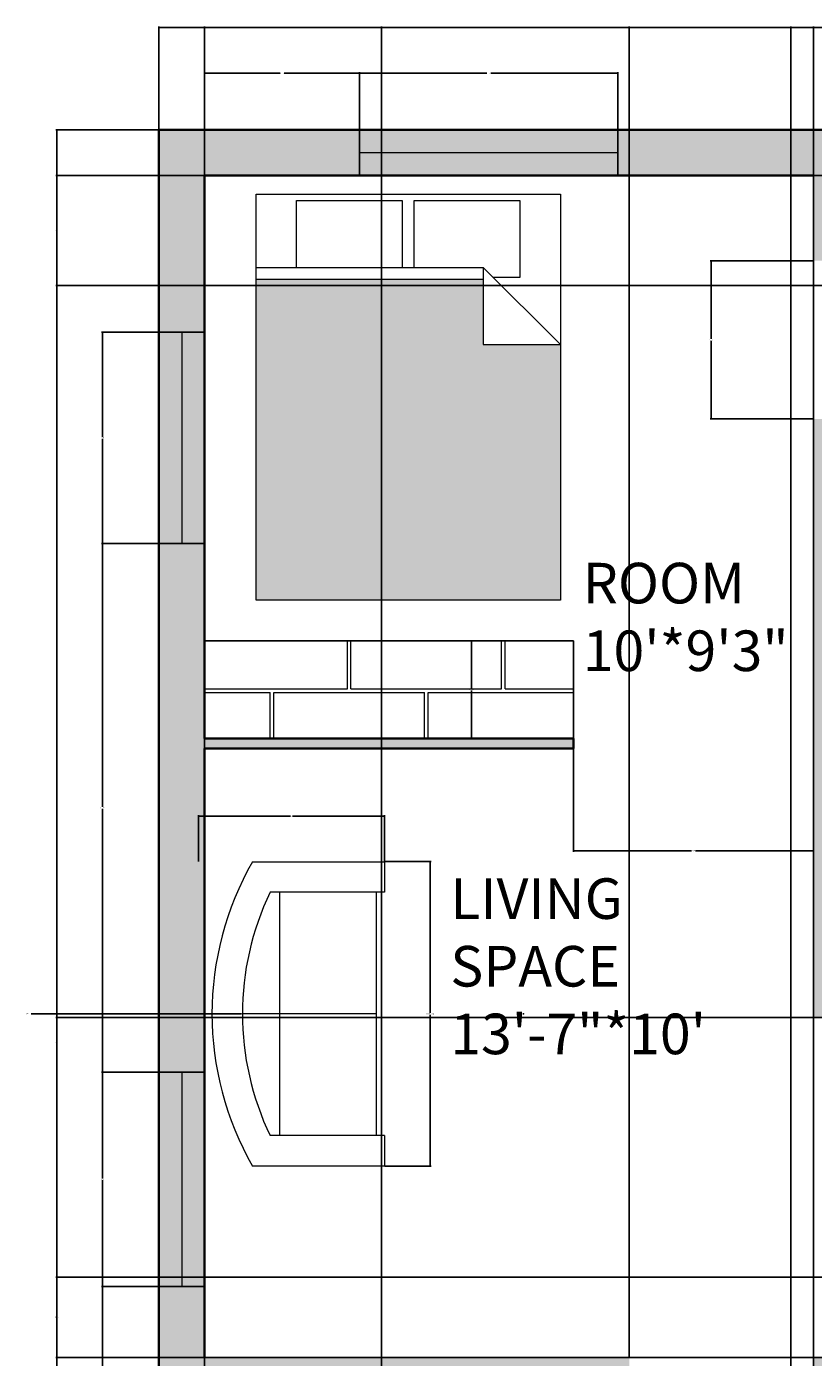
# Model space of a CAD drawing. Units: inches. Extents: x 17031430 to 17032061, y 16082759 to 16083238.
# Tile 2 of 3: x 17031430 to 17031585, y 16082898 to 16083160. Entities that reach past the tile are written whole.
import ezdxf

# ---------------------------------------------------------------- set-up
doc = ezdxf.new("R2010")
doc.units = ezdxf.units.IN
doc.header["$MEASUREMENT"] = 0
for name, color, linetype, lineweight in [('A-ANNO-DIMS', 2, 'Continuous', 18), ('A-AREA-IDEN', 7, 'Continuous', 25), ('A-FLOR-CASE', 8, 'Continuous', 25), ('A-FURN', 8, 'Continuous', 18), ('A-GLAZ', 4, 'Continuous', 18), ('A-WALL', 7, 'Continuous', 35)]:
    doc.layers.add(name, color=color, linetype=linetype, lineweight=lineweight)
for name, color, linetype, lineweight, true_color in [('A-FLOR-CASE-PATT', 9, 'Continuous', 13, 0xc7c8ca), ('A-GLAZ-PATT', 252, 'Continuous', 13, 0x939598), ('A-WALL-PATT', 18, 'Continuous', 13, 0x000000)]:
    doc.layers.add(name, color=color, linetype=linetype, lineweight=lineweight, true_color=true_color)
doc.styles.get("Standard").update_dxf_attribs({"font": 'arial.ttf'})
doc.dimstyles.get("Standard").update_dxf_attribs({"dimtxt": 0.18, "dimasz": 0.18, "dimexe": 0.18, "dimexo": 0.0625, "dimgap": 0.09, "dimtad": 0, "dimtih": 1, "dimtoh": 1, "dimdec": 0, "dimzin": 0, "dimdsep": 46, "dimlunit": 3, "dimtxsty": 'Standard', "dimcen": 0.09, "dimadec": 0, "dimazin": 0, "dimtfac": 1, "dimtdec": 0, "dimtofl": 0, "dimtmove": 0, "dimatfit": 3, "dimfxl": 1, "dimtolj": 1, "dimtzin": 0, "dimarcsym": 0})

# ---------------------------------------------------------------- blocks, each defined once
blk = doc.blocks.new('Bed - Queen')
for p, q in [((0, -80.00003), (0, 0)), ((0, 0), (59.99999, 0)), ((59.99999, 0), (59.99999, -80.00003)), ((7.99999, -1.2), (28.79998, -1.2)), ((7.99999, -14.4), (7.99999, -1.2)), ((28.79998, -1.2), (28.79998, -14.4)), ((31.19999, -1.2), (51.99999, -1.2)), ((31.19999, -14.4), (31.19999, -1.2)), ((51.99999, -1.2), (51.99999, -16.4)), ((0, -14.4), (44.8, -14.4)), ((59.99999, -29.6), (44.8, -14.4)), ((44.8, -14.4), (44.8, -29.6)), ((44.8, -16.8), (0, -16.8)), ((51.99999, -16.4), (46.79936, -16.4)), ((44.8, -29.6), (59.99999, -29.6)), ((59.99999, -80.00003), (0, -80.00003))]:
    blk.add_line(p, q)
blk = doc.blocks.new('Sofa - Roundback Loveseat 5 ft.')
for p, q in [((0, -32.44198), (0, -5.99998)), ((-24, -33.99998), (-24, -11.46958)), ((24.00004, -33.99998), (24.00004, -11.46958)), ((-23.9998, -13.38178), (23.99986, -13.38178)), ((-24, -32.44198), (24.00004, -32.44198))]:
    blk.add_line(p, q)
for points in [[(-24, -33.99998), (-30, -33.99998), (-30, -7.99998)], [(30.00004, -7.99998), (30.00004, -33.99998), (24.00004, -33.99998)]]:
    blk.add_lwpolyline(points)
for centre, radius, start, end in [((0, -60.24998), 60.24998, 60.13715, 119.8628), ((0, -61.38438), 55.38444, 64.32083, 115.6792)]:
    blk.add_arc(centre, radius, start, end)
blk = doc.blocks.new('*D10')
at = {"layer": 'A-ANNO-DIMS', "color": 0, "lineweight": -2, "transparency": 16777216}
for p, q in [((17031500.27, 16082995.46), (17031509.39, 16082995.46)), ((17031509.21, 16082995.28), (17031509.21, 16082965.64)), ((17031509.21, 16082935.64), (17031509.21, 16082965.28)), ((17031500.27, 16082935.46), (17031509.39, 16082935.46))]:
    blk.add_line(p, q, dxfattribs=at)
at = {"layer": 'A-ANNO-DIMS', "color": 0, "transparency": 16777216}
for points in [[(17031509.18, 16082995.28), (17031509.24, 16082995.28), (17031509.21, 16082995.46)], [(17031509.18, 16082935.64), (17031509.24, 16082935.64), (17031509.21, 16082935.46)]]:
    blk.add_solid(points, dxfattribs=at)
at = {"layer": 'Defpoints', "color": 0, "transparency": 16777216}
for p in [(17031500.21, 16082995.46), (17031509.21, 16082995.46), (17031500.21, 16082935.46)]:
    blk.add_point(p, dxfattribs=at)
at = {"layer": 'A-ANNO-DIMS', "color": 0, "transparency": 16777216, "insert": (17031509.21, 16082965.46), "char_height": 0.18, "attachment_point": 5}
blk.add_mtext('\\A1;LOVESEAT 60', dxfattribs=at)
blk = doc.blocks.new('*D11')
at = {"layer": 'A-ANNO-DIMS', "color": 0, "lineweight": -2, "transparency": 16777216}
for p, q in [((17031463.54, 16082995.52), (17031463.54, 16083004.64)), ((17031463.72, 16083004.46), (17031481.66, 16083004.46)), ((17031500.03, 16083004.46), (17031482.09, 16083004.46)), ((17031500.21, 16082995.52), (17031500.21, 16083004.64))]:
    blk.add_line(p, q, dxfattribs=at)
at = {"layer": 'A-ANNO-DIMS', "color": 0, "transparency": 16777216}
for points in [[(17031463.72, 16083004.49), (17031463.72, 16083004.43), (17031463.54, 16083004.46)], [(17031500.03, 16083004.49), (17031500.03, 16083004.43), (17031500.21, 16083004.46)]]:
    blk.add_solid(points, dxfattribs=at)
at = {"layer": 'Defpoints', "color": 0, "transparency": 16777216}
for p in [(17031463.54, 16083004.46), (17031463.54, 16082995.46), (17031500.21, 16082995.46)]:
    blk.add_point(p, dxfattribs=at)
at = {"layer": 'A-ANNO-DIMS', "color": 0, "transparency": 16777216, "insert": (17031481.88, 16083004.46), "char_height": 0.18, "attachment_point": 5}
blk.add_mtext('\\A1;37', dxfattribs=at)
blk = doc.blocks.new('*D14')
at = {"layer": 'A-ANNO-DIMS', "color": 0, "lineweight": -2, "transparency": 16777216}
for p, q in [((17031455.76, 16083139.8), (17031455.76, 16083160.07)), ((17031455.94, 16083159.89), (17031575.47, 16083159.89)), ((17031695.58, 16083159.89), (17031576.05, 16083159.89)), ((17031695.76, 16083139.8), (17031695.76, 16083160.07))]:
    blk.add_line(p, q, dxfattribs=at)
at = {"layer": 'A-ANNO-DIMS', "color": 0, "transparency": 16777216}
for points in [[(17031455.94, 16083159.92), (17031455.94, 16083159.86), (17031455.76, 16083159.89)], [(17031695.58, 16083159.92), (17031695.58, 16083159.86), (17031695.76, 16083159.89)]]:
    blk.add_solid(points, dxfattribs=at)
at = {"layer": 'Defpoints', "color": 0, "transparency": 16777216}
for p in [(17031695.76, 16083159.89), (17031455.76, 16083139.74), (17031695.76, 16083139.74)]:
    blk.add_point(p, dxfattribs=at)
at = {"layer": 'A-ANNO-DIMS', "color": 0, "transparency": 16777216, "insert": (17031575.76, 16083159.89), "char_height": 0.18, "attachment_point": 5}
blk.add_mtext('\\A1;240', dxfattribs=at)
blk = doc.blocks.new('*D15')
at = {"layer": 'A-ANNO-DIMS', "color": 0, "lineweight": -2, "transparency": 16777216}
for p, q in [((17031455.69, 16083139.74), (17031435.43, 16083139.74)), ((17031435.61, 16083139.56), (17031435.61, 16082959.92)), ((17031435.61, 16082779.92), (17031435.61, 16082959.56)), ((17031455.69, 16082779.74), (17031435.43, 16082779.74))]:
    blk.add_line(p, q, dxfattribs=at)
at = {"layer": 'A-ANNO-DIMS', "color": 0, "transparency": 16777216}
for points in [[(17031435.58, 16083139.56), (17031435.64, 16083139.56), (17031435.61, 16083139.74)], [(17031435.58, 16082779.92), (17031435.64, 16082779.92), (17031435.61, 16082779.74)]]:
    blk.add_solid(points, dxfattribs=at)
at = {"layer": 'Defpoints', "color": 0, "transparency": 16777216}
for p in [(17031435.61, 16083139.74), (17031455.76, 16083139.74), (17031455.76, 16082779.74)]:
    blk.add_point(p, dxfattribs=at)
at = {"layer": 'A-ANNO-DIMS', "color": 0, "transparency": 16777216, "insert": (17031435.61, 16082959.74), "char_height": 0.18, "attachment_point": 5}
blk.add_mtext('\\A1;360', dxfattribs=at)
blk = doc.blocks.new('*D16')
at = {"layer": 'A-ANNO-DIMS', "color": 0, "lineweight": -2, "transparency": 16777216}
for p, q in [((17031464.76, 16083130.8), (17031464.76, 16083151.07)), ((17031464.94, 16083150.89), (17031479.63, 16083150.89)), ((17031495.11, 16083150.89), (17031480.42, 16083150.89)), ((17031495.29, 16083130.8), (17031495.29, 16083151.07))]:
    blk.add_line(p, q, dxfattribs=at)
at = {"layer": 'A-ANNO-DIMS', "color": 0, "transparency": 16777216}
for points in [[(17031464.94, 16083150.92), (17031464.94, 16083150.86), (17031464.76, 16083150.89)], [(17031495.11, 16083150.92), (17031495.11, 16083150.86), (17031495.29, 16083150.89)]]:
    blk.add_solid(points, dxfattribs=at)
at = {"layer": 'Defpoints', "color": 0, "transparency": 16777216}
for p in [(17031495.29, 16083150.89), (17031464.76, 16083130.74), (17031495.29, 16083130.74)]:
    blk.add_point(p, dxfattribs=at)
at = {"layer": 'A-ANNO-DIMS', "color": 0, "transparency": 16777216, "insert": (17031480.02, 16083150.89), "char_height": 0.18, "attachment_point": 5}
blk.add_mtext('\\A1;30.53', dxfattribs=at)
blk = doc.blocks.new('*D17')
at = {"layer": 'A-ANNO-DIMS', "color": 0, "lineweight": -2, "transparency": 16777216}
for p, q in [((17031495.29, 16083130.8), (17031495.29, 16083151.07)), ((17031495.47, 16083150.89), (17031520.36, 16083150.89)), ((17031546.04, 16083150.89), (17031521.15, 16083150.89)), ((17031546.22, 16083130.8), (17031546.22, 16083151.07))]:
    blk.add_line(p, q, dxfattribs=at)
at = {"layer": 'A-ANNO-DIMS', "color": 0, "transparency": 16777216}
for points in [[(17031495.47, 16083150.92), (17031495.47, 16083150.86), (17031495.29, 16083150.89)], [(17031546.04, 16083150.92), (17031546.04, 16083150.86), (17031546.22, 16083150.89)]]:
    blk.add_solid(points, dxfattribs=at)
at = {"layer": 'Defpoints', "color": 0, "transparency": 16777216}
for p in [(17031546.22, 16083150.89), (17031495.29, 16083130.74), (17031546.22, 16083130.74)]:
    blk.add_point(p, dxfattribs=at)
at = {"layer": 'A-ANNO-DIMS', "color": 0, "transparency": 16777216, "insert": (17031520.76, 16083150.89), "char_height": 0.18, "attachment_point": 5}
blk.add_mtext('\\A1;50.94', dxfattribs=at)
blk = doc.blocks.new('*D23')
at = {"layer": 'A-ANNO-DIMS', "color": 0, "lineweight": -2, "transparency": 16777216}
for p, q in [((17031464.69, 16082911.7), (17031444.43, 16082911.7)), ((17031444.61, 16082911.52), (17031444.61, 16082887.51)), ((17031444.61, 16082863.13), (17031444.61, 16082887.14)), ((17031464.69, 16082862.95), (17031444.43, 16082862.95))]:
    blk.add_line(p, q, dxfattribs=at)
at = {"layer": 'A-ANNO-DIMS', "color": 0, "transparency": 16777216}
for points in [[(17031444.58, 16082911.52), (17031444.64, 16082911.52), (17031444.61, 16082911.7)], [(17031444.58, 16082863.13), (17031444.64, 16082863.13), (17031444.61, 16082862.95)]]:
    blk.add_solid(points, dxfattribs=at)
at = {"layer": 'Defpoints', "color": 0, "transparency": 16777216}
for p in [(17031444.61, 16082911.7), (17031464.76, 16082911.7), (17031464.76, 16082862.95)]:
    blk.add_point(p, dxfattribs=at)
at = {"layer": 'A-ANNO-DIMS', "color": 0, "transparency": 16777216, "insert": (17031444.61, 16082887.33), "char_height": 0.18, "attachment_point": 5}
blk.add_mtext('\\A1;48.74', dxfattribs=at)
blk = doc.blocks.new('*D24')
at = {"layer": 'A-ANNO-DIMS', "color": 0, "lineweight": -2, "transparency": 16777216}
for p, q in [((17031464.69, 16082953.98), (17031444.43, 16082953.98)), ((17031444.61, 16082953.8), (17031444.61, 16082933.02)), ((17031444.61, 16082911.88), (17031444.61, 16082932.66)), ((17031464.69, 16082911.7), (17031444.43, 16082911.7))]:
    blk.add_line(p, q, dxfattribs=at)
at = {"layer": 'A-ANNO-DIMS', "color": 0, "transparency": 16777216}
for points in [[(17031444.58, 16082953.8), (17031444.64, 16082953.8), (17031444.61, 16082953.98)], [(17031444.58, 16082911.88), (17031444.64, 16082911.88), (17031444.61, 16082911.7)]]:
    blk.add_solid(points, dxfattribs=at)
at = {"layer": 'Defpoints', "color": 0, "transparency": 16777216}
for p in [(17031444.61, 16082953.98), (17031464.76, 16082953.98), (17031464.76, 16082911.7)]:
    blk.add_point(p, dxfattribs=at)
at = {"layer": 'A-ANNO-DIMS', "color": 0, "transparency": 16777216, "insert": (17031444.61, 16082932.84), "char_height": 0.18, "attachment_point": 5}
blk.add_mtext('\\A1;42.28', dxfattribs=at)
blk = doc.blocks.new('*D25')
at = {"layer": 'A-ANNO-DIMS', "color": 0, "lineweight": -2, "transparency": 16777216}
for p, q in [((17031464.69, 16083058.17), (17031444.43, 16083058.17)), ((17031444.61, 16083057.99), (17031444.61, 16083006.26)), ((17031444.61, 16082954.16), (17031444.61, 16083005.89)), ((17031464.69, 16082953.98), (17031444.43, 16082953.98))]:
    blk.add_line(p, q, dxfattribs=at)
at = {"layer": 'A-ANNO-DIMS', "color": 0, "transparency": 16777216}
for points in [[(17031444.58, 16083057.99), (17031444.64, 16083057.99), (17031444.61, 16083058.17)], [(17031444.58, 16082954.16), (17031444.64, 16082954.16), (17031444.61, 16082953.98)]]:
    blk.add_solid(points, dxfattribs=at)
at = {"layer": 'Defpoints', "color": 0, "transparency": 16777216}
for p in [(17031444.61, 16083058.17), (17031464.76, 16083058.17), (17031464.76, 16082953.98)]:
    blk.add_point(p, dxfattribs=at)
at = {"layer": 'A-ANNO-DIMS', "color": 0, "transparency": 16777216, "insert": (17031444.61, 16083006.07), "char_height": 0.18, "attachment_point": 5}
blk.add_mtext('\\A1;104.19', dxfattribs=at)
blk = doc.blocks.new('*D26')
at = {"layer": 'A-ANNO-DIMS', "color": 0, "lineweight": -2, "transparency": 16777216}
for p, q in [((17031464.69, 16083099.83), (17031444.43, 16083099.83)), ((17031444.61, 16083099.65), (17031444.61, 16083079.18)), ((17031444.61, 16083058.35), (17031444.61, 16083078.82)), ((17031464.69, 16083058.17), (17031444.43, 16083058.17))]:
    blk.add_line(p, q, dxfattribs=at)
at = {"layer": 'A-ANNO-DIMS', "color": 0, "transparency": 16777216}
for points in [[(17031444.58, 16083099.65), (17031444.64, 16083099.65), (17031444.61, 16083099.83)], [(17031444.58, 16083058.35), (17031444.64, 16083058.35), (17031444.61, 16083058.17)]]:
    blk.add_solid(points, dxfattribs=at)
at = {"layer": 'Defpoints', "color": 0, "transparency": 16777216}
for p in [(17031444.61, 16083099.83), (17031464.76, 16083099.83), (17031464.76, 16083058.17)]:
    blk.add_point(p, dxfattribs=at)
at = {"layer": 'A-ANNO-DIMS', "color": 0, "transparency": 16777216, "insert": (17031444.61, 16083079), "char_height": 0.18, "attachment_point": 5}
blk.add_mtext('\\A1;41.66', dxfattribs=at)
blk = doc.blocks.new('*D38')
at = {"layer": 'A-ANNO-DIMS', "color": 0, "lineweight": -2, "transparency": 16777216}
for p, q in [((17031537.5, 16083017.68), (17031537.5, 16082997.41)), ((17031584.76, 16083017.68), (17031584.76, 16082997.41)), ((17031537.68, 16082997.59), (17031560.73, 16082997.59)), ((17031584.58, 16082997.59), (17031561.53, 16082997.59))]:
    blk.add_line(p, q, dxfattribs=at)
at = {"layer": 'A-ANNO-DIMS', "color": 0, "transparency": 16777216}
for points in [[(17031537.68, 16082997.62), (17031537.68, 16082997.56), (17031537.5, 16082997.59)], [(17031584.58, 16082997.62), (17031584.58, 16082997.56), (17031584.76, 16082997.59)]]:
    blk.add_solid(points, dxfattribs=at)
at = {"layer": 'Defpoints', "color": 0, "transparency": 16777216}
for p in [(17031537.5, 16083017.74), (17031584.76, 16083017.74), (17031537.5, 16082997.59)]:
    blk.add_point(p, dxfattribs=at)
at = {"layer": 'A-ANNO-DIMS', "color": 0, "transparency": 16777216, "insert": (17031561.13, 16082997.59), "char_height": 0.18, "attachment_point": 5}
blk.add_mtext('\\A1;47.26', dxfattribs=at)
blk = doc.blocks.new('*D39')
at = {"layer": 'A-ANNO-DIMS', "color": 0, "lineweight": -2, "transparency": 16777216}
for p, q in [((17031548.47, 16082897.8), (17031548.47, 16083160.07)), ((17031548.65, 16083159.89), (17031566.22, 16083159.89)), ((17031584.58, 16083159.89), (17031567.01, 16083159.89)), ((17031584.76, 16082897.8), (17031584.76, 16083160.07))]:
    blk.add_line(p, q, dxfattribs=at)
at = {"layer": 'A-ANNO-DIMS', "color": 0, "transparency": 16777216}
for points in [[(17031548.65, 16083159.92), (17031548.65, 16083159.86), (17031548.47, 16083159.89)], [(17031584.58, 16083159.92), (17031584.58, 16083159.86), (17031584.76, 16083159.89)]]:
    blk.add_solid(points, dxfattribs=at)
at = {"layer": 'Defpoints', "color": 0, "transparency": 16777216}
for p in [(17031584.76, 16083159.89), (17031548.47, 16082897.74), (17031584.76, 16082897.74)]:
    blk.add_point(p, dxfattribs=at)
at = {"layer": 'A-ANNO-DIMS', "color": 0, "transparency": 16777216, "insert": (17031566.61, 16083159.89), "char_height": 0.18, "attachment_point": 5}
blk.add_mtext('\\A1;36.29', dxfattribs=at)
blk = doc.blocks.new('*D41')
at = {"layer": 'A-ANNO-DIMS', "color": 0, "lineweight": -2, "transparency": 16777216}
for p, q in [((17031584.69, 16083113.92), (17031564.43, 16083113.92)), ((17031564.61, 16083113.74), (17031564.61, 16083098.51)), ((17031564.61, 16083082.92), (17031564.61, 16083098.15)), ((17031584.69, 16083082.74), (17031564.43, 16083082.74))]:
    blk.add_line(p, q, dxfattribs=at)
at = {"layer": 'A-ANNO-DIMS', "color": 0, "transparency": 16777216}
for points in [[(17031564.58, 16083113.74), (17031564.64, 16083113.74), (17031564.61, 16083113.92)], [(17031564.58, 16083082.92), (17031564.64, 16083082.92), (17031564.61, 16083082.74)]]:
    blk.add_solid(points, dxfattribs=at)
at = {"layer": 'Defpoints', "color": 0, "transparency": 16777216}
for p in [(17031564.61, 16083113.92), (17031584.76, 16083113.92), (17031584.76, 16083082.74)]:
    blk.add_point(p, dxfattribs=at)
at = {"layer": 'A-ANNO-DIMS', "color": 0, "transparency": 16777216, "insert": (17031564.61, 16083098.33), "char_height": 0.18, "attachment_point": 5}
blk.add_mtext('\\A1;31.176', dxfattribs=at)
blk = doc.blocks.new('*D44')
at = {"layer": 'A-ANNO-DIMS', "color": 0, "lineweight": -2, "transparency": 16777216}
for p, q in [((17031630.06, 16082964.74), (17031435.43, 16082964.74)), ((17031435.61, 16082964.56), (17031435.61, 16082931.42)), ((17031435.61, 16082897.92), (17031435.61, 16082931.06)), ((17031629.85, 16082897.74), (17031435.43, 16082897.74))]:
    blk.add_line(p, q, dxfattribs=at)
at = {"layer": 'A-ANNO-DIMS', "color": 0, "transparency": 16777216}
for points in [[(17031435.58, 16082964.56), (17031435.64, 16082964.56), (17031435.61, 16082964.74)], [(17031435.58, 16082897.92), (17031435.64, 16082897.92), (17031435.61, 16082897.74)]]:
    blk.add_solid(points, dxfattribs=at)
at = {"layer": 'Defpoints', "color": 0, "transparency": 16777216}
for p in [(17031435.61, 16082964.74), (17031630.12, 16082964.74), (17031629.91, 16082897.74)]:
    blk.add_point(p, dxfattribs=at)
at = {"layer": 'A-ANNO-DIMS', "color": 0, "transparency": 16777216, "insert": (17031435.61, 16082931.24), "char_height": 0.18, "attachment_point": 5}
blk.add_mtext('\\A1;67', dxfattribs=at)
blk = doc.blocks.new('*D45')
at = {"layer": 'A-ANNO-DIMS', "color": 0, "lineweight": -2, "transparency": 16777216}
for p, q in [((17031464.76, 16082895.8), (17031464.76, 16083160.07)), ((17031464.94, 16083159.89), (17031481.79, 16083159.89)), ((17031499.44, 16083159.89), (17031482.58, 16083159.89)), ((17031499.62, 16082895.8), (17031499.62, 16083160.07))]:
    blk.add_line(p, q, dxfattribs=at)
at = {"layer": 'A-ANNO-DIMS', "color": 0, "transparency": 16777216}
for points in [[(17031464.94, 16083159.92), (17031464.94, 16083159.86), (17031464.76, 16083159.89)], [(17031499.44, 16083159.92), (17031499.44, 16083159.86), (17031499.62, 16083159.89)]]:
    blk.add_solid(points, dxfattribs=at)
at = {"layer": 'Defpoints', "color": 0, "transparency": 16777216}
for p in [(17031499.62, 16083159.89), (17031464.76, 16082895.74), (17031499.62, 16082895.74)]:
    blk.add_point(p, dxfattribs=at)
at = {"layer": 'A-ANNO-DIMS', "color": 0, "transparency": 16777216, "insert": (17031482.19, 16083159.89), "char_height": 0.18, "attachment_point": 5}
blk.add_mtext('\\A1;34.86', dxfattribs=at)
blk = doc.blocks.new('*D47')
at = {"layer": 'A-ANNO-DIMS', "color": 0, "lineweight": -2, "transparency": 16777216}
for p, q in [((17031580.32, 16082820.21), (17031580.32, 16083160.07)), ((17031580.5, 16083159.89), (17031582.16, 16083159.89)), ((17031584.58, 16083159.89), (17031582.92, 16083159.89)), ((17031584.76, 16082820.21), (17031584.76, 16083160.07))]:
    blk.add_line(p, q, dxfattribs=at)
at = {"layer": 'A-ANNO-DIMS', "color": 0, "transparency": 16777216}
for points in [[(17031580.5, 16083159.92), (17031580.5, 16083159.86), (17031580.32, 16083159.89)], [(17031584.58, 16083159.92), (17031584.58, 16083159.86), (17031584.76, 16083159.89)]]:
    blk.add_solid(points, dxfattribs=at)
at = {"layer": 'Defpoints', "color": 0, "transparency": 16777216}
for p in [(17031584.76, 16083159.89), (17031580.32, 16082820.15), (17031584.76, 16082820.15)]:
    blk.add_point(p, dxfattribs=at)
at = {"layer": 'A-ANNO-DIMS', "color": 0, "transparency": 16777216, "insert": (17031582.54, 16083159.89), "char_height": 0.18, "attachment_point": 5}
blk.add_mtext('\\A1;4.441', dxfattribs=at)
blk = doc.blocks.new('*D51')
at = {"layer": 'A-ANNO-DIMS', "color": 0, "lineweight": -2, "transparency": 16777216}
for p, q in [((17031537.44, 16083038.98), (17031517.17, 16083038.98)), ((17031517.35, 16083038.8), (17031517.35, 16083029.54)), ((17031517.35, 16083019.92), (17031517.35, 16083029.18)), ((17031537.44, 16083019.74), (17031517.17, 16083019.74))]:
    blk.add_line(p, q, dxfattribs=at)
at = {"layer": 'A-ANNO-DIMS', "color": 0, "transparency": 16777216}
for points in [[(17031517.32, 16083038.8), (17031517.38, 16083038.8), (17031517.35, 16083038.98)], [(17031517.32, 16083019.92), (17031517.38, 16083019.92), (17031517.35, 16083019.74)]]:
    blk.add_solid(points, dxfattribs=at)
at = {"layer": 'Defpoints', "color": 0, "transparency": 16777216}
for p in [(17031517.35, 16083038.98), (17031537.5, 16083038.98), (17031537.5, 16083019.74)]:
    blk.add_point(p, dxfattribs=at)
at = {"layer": 'A-ANNO-DIMS', "color": 0, "transparency": 16777216, "insert": (17031517.35, 16083029.36), "char_height": 0.18, "attachment_point": 5}
blk.add_mtext('\\A1;19.236', dxfattribs=at)
blk = doc.blocks.new('*D53')
at = {"layer": 'A-ANNO-DIMS', "color": 0, "lineweight": -2, "transparency": 16777216}
for p, q in [((17031654.72, 16082913.56), (17031435.43, 16082913.56)), ((17031435.61, 16082913.38), (17031435.61, 16082905.83)), ((17031435.61, 16082897.92), (17031435.61, 16082905.47)), ((17031686.69, 16082897.74), (17031435.43, 16082897.74))]:
    blk.add_line(p, q, dxfattribs=at)
at = {"layer": 'A-ANNO-DIMS', "color": 0, "transparency": 16777216}
for points in [[(17031435.58, 16082913.38), (17031435.64, 16082913.38), (17031435.61, 16082913.56)], [(17031435.58, 16082897.92), (17031435.64, 16082897.92), (17031435.61, 16082897.74)]]:
    blk.add_solid(points, dxfattribs=at)
at = {"layer": 'Defpoints', "color": 0, "transparency": 16777216}
for p in [(17031435.61, 16082913.56), (17031654.78, 16082913.56), (17031686.76, 16082897.74)]:
    blk.add_point(p, dxfattribs=at)
at = {"layer": 'A-ANNO-DIMS', "color": 0, "transparency": 16777216, "insert": (17031435.61, 16082905.65), "char_height": 0.18, "attachment_point": 5}
blk.add_mtext('\\A1;15.824', dxfattribs=at)
blk = doc.blocks.new('*D55')
at = {"layer": 'A-ANNO-DIMS', "color": 0, "lineweight": -2, "transparency": 16777216}
for p, q in [((17031686.69, 16083130.74), (17031435.43, 16083130.74)), ((17031435.61, 16083130.56), (17031435.61, 16083120.07)), ((17031435.61, 16083109.22), (17031435.61, 16083119.71)), ((17031655.38, 16083109.04), (17031435.43, 16083109.04))]:
    blk.add_line(p, q, dxfattribs=at)
at = {"layer": 'A-ANNO-DIMS', "color": 0, "transparency": 16777216}
for points in [[(17031435.58, 16083130.56), (17031435.64, 16083130.56), (17031435.61, 16083130.74)], [(17031435.58, 16083109.22), (17031435.64, 16083109.22), (17031435.61, 16083109.04)]]:
    blk.add_solid(points, dxfattribs=at)
at = {"layer": 'Defpoints', "color": 0, "transparency": 16777216}
for p in [(17031686.76, 16083130.74), (17031435.61, 16083109.04), (17031655.44, 16083109.04)]:
    blk.add_point(p, dxfattribs=at)
at = {"layer": 'A-ANNO-DIMS', "color": 0, "transparency": 16777216, "insert": (17031435.61, 16083119.89), "char_height": 0.18, "attachment_point": 5}
blk.add_mtext('\\A1;21.7', dxfattribs=at)
blk = doc.blocks.new('*D56')
at = {"layer": 'A-ANNO-DIMS', "color": 0, "lineweight": -2, "transparency": 16777216}
for p, q in [((17031430.54, 16082965.46), (17031466.03, 16082965.46)), ((17031526.37, 16082965.46), (17031526.55, 16082965.46)), ((17031526.46, 16082965.37), (17031526.46, 16082965.55))]:
    blk.add_line(p, q, dxfattribs=at)
at = {"layer": 'A-ANNO-DIMS', "color": 0, "transparency": 16777216}
blk.add_solid([(17031466.03, 16082965.49), (17031466.03, 16082965.43), (17031466.21, 16082965.46)], dxfattribs=at)
at = {"layer": 'Defpoints', "color": 0, "transparency": 16777216}
for p in [(17031466.21, 16082965.46), (17031526.46, 16082965.46)]:
    blk.add_point(p, dxfattribs=at)
at = {"layer": 'A-ANNO-DIMS', "color": 0, "transparency": 16777216, "insert": (17031430.06, 16082965.46), "char_height": 0.18, "attachment_point": 5}
blk.add_mtext('\\A1;R60.25', dxfattribs=at)
blk = doc.blocks.new('*D57')
at = {"layer": 'A-ANNO-DIMS', "color": 0, "lineweight": -2, "transparency": 16777216}
for p, q in [((17031439.46, 16082965.46), (17031472.03, 16082965.46)), ((17031527.5, 16082965.46), (17031527.68, 16082965.46)), ((17031527.59, 16082965.37), (17031527.59, 16082965.55))]:
    blk.add_line(p, q, dxfattribs=at)
at = {"layer": 'A-ANNO-DIMS', "color": 0, "transparency": 16777216}
blk.add_solid([(17031472.03, 16082965.49), (17031472.03, 16082965.43), (17031472.21, 16082965.46)], dxfattribs=at)
at = {"layer": 'Defpoints', "color": 0, "transparency": 16777216}
for p in [(17031472.21, 16082965.46), (17031527.59, 16082965.46)]:
    blk.add_point(p, dxfattribs=at)
at = {"layer": 'A-ANNO-DIMS', "color": 0, "transparency": 16777216, "insert": (17031438.98, 16082965.46), "char_height": 0.18, "attachment_point": 5}
blk.add_mtext('\\A1;R55.38', dxfattribs=at)

msp = doc.modelspace()

# ---------------------------------------------------------------- hatches: boundary and pattern name
at = {"layer": 'A-FLOR-CASE-PATT'}
h = msp.add_hatch(dxfattribs=at)
h.set_pattern_fill('AR-B816C', color=256, scale=1.9)
h.paths.add_polyline_path([(17031537.499, 16083038.9761), (17031464.7571, 16083038.9761), (17031464.7571, 16083019.7405), (17031537.499, 16083019.7405)])
at = {"layer": 'A-GLAZ-PATT'}
h = msp.add_hatch(color=256, dxfattribs=at)
h.dxf.hatch_style = 1
h.paths.add_polyline_path([(17031546.2248, 16083139.7405), (17031495.2896, 16083139.7405), (17031495.2896, 16083135.2405), (17031546.2248, 16083135.2405)])
h.paths.add_polyline_path([(17031546.2248, 16083135.2405), (17031495.2896, 16083135.2405), (17031495.2896, 16083130.7405), (17031546.2248, 16083130.7405)])
h.paths.add_polyline_path([(17031464.7571, 16083099.8263), (17031460.2571, 16083099.8263), (17031460.2571, 16083058.1685), (17031464.7571, 16083058.1685)])
h.paths.add_polyline_path([(17031460.2571, 16083099.8263), (17031455.7571, 16083099.8263), (17031455.7571, 16083058.1685), (17031460.2571, 16083058.1685)])
h.paths.add_polyline_path([(17031464.7571, 16082953.9805), (17031460.2571, 16082953.9805), (17031460.2571, 16082911.6971), (17031464.7571, 16082911.6971)])
h.paths.add_polyline_path([(17031460.2571, 16082953.9805), (17031455.7571, 16082953.9805), (17031455.7571, 16082911.6971), (17031460.2571, 16082911.6971)])
h.paths.add_polyline_path([(17031460.2571, 16082862.954), (17031455.7571, 16082862.954), (17031455.7571, 16082807.1802), (17031460.2571, 16082807.1802)])
h.paths.add_polyline_path([(17031464.7571, 16082862.954), (17031460.2571, 16082862.954), (17031460.2571, 16082807.1802), (17031464.7571, 16082807.1802)])
h.paths.add_polyline_path([(17031681.0952, 16082784.2405), (17031647.5287, 16082784.2405), (17031647.5287, 16082779.7405), (17031681.0952, 16082779.7405)])
h.paths.add_polyline_path([(17031681.0952, 16082788.7405), (17031647.5287, 16082788.7405), (17031647.5287, 16082784.2405), (17031681.0952, 16082784.2405)])
h.paths.add_polyline_path([(17031691.2571, 16083057.4652), (17031686.7571, 16083057.4652), (17031686.7571, 16083009.0162), (17031691.2571, 16083009.0162)])
h.paths.add_polyline_path([(17031514.2108, 16082846.7675), (17031567.264, 16082846.7675), (17031567.264, 16082876.6193), (17031514.2108, 16082876.6193)], flags=9)
h.paths.add_polyline_path([(17031636.4861, 16082934.711), (17031688.115, 16082934.711), (17031688.115, 16082964.5628), (17031636.4861, 16082964.5628)], flags=9)
h.paths.add_polyline_path([(17031509.9735, 16082952.8397), (17031561.3568, 16082952.8397), (17031561.3568, 16082996.1612), (17031509.9735, 16082996.1612)], flags=9)
h.paths.add_polyline_path([(17031605.4082, 16082988.2134), (17031667.1545, 16082988.2134), (17031667.1545, 16083004.6991), (17031605.4082, 16083004.6991)], flags=9)
h.paths.add_polyline_path([(17031598.2513, 16083096.6971), (17031641.5746, 16083096.6971), (17031641.5746, 16083126.5489), (17031598.2513, 16083126.5489)], flags=9)
h.paths.add_polyline_path([(17031536.0858, 16083028.4916), (17031577.5319, 16083028.4916), (17031577.5319, 16083058.3434), (17031536.0858, 16083058.3434)], flags=9)
h = msp.add_hatch(color=256, dxfattribs=at)
h.dxf.hatch_style = 1
h.paths.add_polyline_path([(17031695.7571, 16083124.4975), (17031691.2571, 16083124.4975), (17031691.2571, 16083092.6946), (17031695.7571, 16083092.6946)])
h.paths.add_polyline_path([(17031691.2571, 16083124.4975), (17031686.7571, 16083124.4975), (17031686.7571, 16083092.6946), (17031691.2571, 16083092.6946)])
h.paths.add_polyline_path([(17031695.7571, 16083057.4652), (17031691.2571, 16083057.4652), (17031691.2571, 16083009.0162), (17031695.7571, 16083009.0162)])
h.paths.add_polyline_path([(17031534.8905, 16083097.4163), (17031519.6905, 16083097.4163), (17031519.6905, 16083110.2163), (17031474.8905, 16083110.2163), (17031474.8905, 16083047.0163), (17031534.8905, 16083047.0163)])
h.paths.add_polyline_path([(17031670.1648, 16083077.6823), (17031619.7648, 16083077.6823), (17031619.7648, 16083062.4823), (17031606.9648, 16083062.4823), (17031606.9648, 16083017.6823), (17031670.1648, 16083017.6823)])
at = {"layer": 'A-WALL-PATT'}
h = msp.add_hatch(color=256, dxfattribs=at)
h.dxf.hatch_style = 1
h.paths.add_polyline_path([(17031695.7571, 16083009.0162), (17031686.7571, 16083009.0162), (17031686.7571, 16082966.7405), (17031630.1205, 16082966.7405), (17031630.1205, 16082964.7405), (17031686.7571, 16082964.7405), (17031686.7571, 16082936.7854), (17031695.7571, 16082936.7854)])
h.paths.add_polyline_path([(17031695.7571, 16083092.6946), (17031686.7571, 16083092.6946), (17031686.7571, 16083082.7405), (17031584.7571, 16083082.7405), (17031584.7571, 16083019.7405), (17031584.7571, 16083017.7405), (17031584.7571, 16082966.7405), (17031584.7571, 16082964.7405), (17031586.7571, 16082964.7405), (17031586.7571, 16082966.7405), (17031586.7571, 16083080.7405), (17031686.7571, 16083080.7405), (17031686.7571, 16083057.4652), (17031695.7571, 16083057.4652)])
h.paths.add_polyline_path([(17031695.7571, 16083139.7405), (17031546.2248, 16083139.7405), (17031546.2248, 16083130.7405), (17031584.7571, 16083130.7405), (17031584.7571, 16083113.9162), (17031586.7571, 16083113.9162), (17031586.7571, 16083130.7405), (17031686.7571, 16083130.7405), (17031686.7571, 16083124.4975), (17031695.7571, 16083124.4975)])
h.paths.add_polyline_path([(17031495.2896, 16083139.7405), (17031455.7571, 16083139.7405), (17031455.7571, 16083099.8263), (17031464.7571, 16083099.8263), (17031464.7571, 16083130.7405), (17031495.2896, 16083130.7405)])
h.paths.add_polyline_path([(17031537.499, 16083019.7405), (17031464.7571, 16083019.7405), (17031464.7571, 16083058.1685), (17031455.7571, 16083058.1685), (17031455.7571, 16082953.9805), (17031464.7571, 16082953.9805), (17031464.7571, 16083017.7405), (17031537.499, 16083017.7405)])
h.paths.add_polyline_path([(17031464.7571, 16082911.6971), (17031455.7571, 16082911.6971), (17031455.7571, 16082862.954), (17031464.7571, 16082862.954), (17031464.7571, 16082895.7405), (17031548.467, 16082895.7405), (17031548.467, 16082897.7405), (17031464.7571, 16082897.7405)])
h.paths.add_polyline_path([(17031464.7571, 16082807.1802), (17031455.7571, 16082807.1802), (17031455.7571, 16082779.7405), (17031647.5287, 16082779.7405), (17031647.5287, 16082788.7405), (17031586.7571, 16082788.7405), (17031586.7571, 16082897.7405), (17031584.7571, 16082897.7405), (17031584.7571, 16082895.7405), (17031584.7571, 16082788.7405), (17031464.7571, 16082788.7405)])
h.paths.add_polyline_path([(17031514.2108, 16082846.7675), (17031567.264, 16082846.7675), (17031567.264, 16082876.6193), (17031514.2108, 16082876.6193)], flags=25)
h.paths.add_polyline_path([(17031636.4861, 16082934.711), (17031688.115, 16082934.711), (17031688.115, 16082964.5628), (17031636.4861, 16082964.5628)], flags=9)
h.paths.add_polyline_path([(17031509.9735, 16082952.8397), (17031561.3568, 16082952.8397), (17031561.3568, 16082996.1612), (17031509.9735, 16082996.1612)], flags=9)
h.paths.add_polyline_path([(17031605.4082, 16082988.2134), (17031667.1545, 16082988.2134), (17031667.1545, 16083004.6991), (17031605.4082, 16083004.6991)], flags=25)
h.paths.add_polyline_path([(17031598.2513, 16083096.6971), (17031641.5746, 16083096.6971), (17031641.5746, 16083126.5489), (17031598.2513, 16083126.5489)], flags=9)
h.paths.add_polyline_path([(17031536.0858, 16083028.4916), (17031577.5319, 16083028.4916), (17031577.5319, 16083058.3434), (17031536.0858, 16083058.3434)], flags=9)

# ---------------------------------------------------------------- linework, layer by layer
at = {"layer": 'A-FLOR-CASE'}
for p, q in [((17031537.499, 16083038.9761), (17031464.7571, 16083038.9761)), ((17031537.499, 16083019.7405), (17031537.499, 16083038.9761))]:
    msp.add_line(p, q, dxfattribs=at)
at = {"layer": 'A-GLAZ'}
for p, q in [((17031495.2896, 16083139.7405), (17031495.2896, 16083130.7405)), ((17031546.2248, 16083139.7405), (17031546.2248, 16083130.7405)), ((17031495.2896, 16083135.2405), (17031546.2248, 16083135.2405)), ((17031455.7571, 16083099.8263), (17031464.7571, 16083099.8263)), ((17031460.2571, 16083099.8263), (17031460.2571, 16083058.1685)), ((17031455.7571, 16083058.1685), (17031464.7571, 16083058.1685)), ((17031455.7571, 16082953.9805), (17031464.7571, 16082953.9805)), ((17031460.2571, 16082953.9805), (17031460.2571, 16082911.6971)), ((17031455.7571, 16082911.6971), (17031464.7571, 16082911.6971))]:
    msp.add_line(p, q, dxfattribs=at)
at = {"layer": 'A-WALL'}
for p, q in [((17031464.7571, 16083130.7405), (17031584.7571, 16083130.7405)), ((17031464.7571, 16083019.7405), (17031464.7571, 16083130.7405)), ((17031464.7571, 16083019.7405), (17031537.499, 16083019.7405)), ((17031537.499, 16083019.7405), (17031537.499, 16083017.7405)), ((17031464.7571, 16083017.7405), (17031537.499, 16083017.7405)), ((17031464.7571, 16082897.7405), (17031464.7571, 16083017.7405))]:
    msp.add_line(p, q, dxfattribs=at)
msp.add_lwpolyline([(17031695.7571, 16082779.7405), (17031455.7571, 16082779.7405), (17031455.7571, 16083139.7405), (17031695.7571, 16083139.7405)], close=True, dxfattribs=at)

# ---------------------------------------------------------------- block references
at = {"layer": 'A-FURN'}
msp.add_blockref('Bed - Queen', (17031474.8905, 16083127.0163), dxfattribs=at)
at = {"layer": 'A-FURN', "rotation": 89.99974895413732}
msp.add_blockref('Sofa - Roundback Loveseat 5 ft.', (17031466.2083, 16082965.4593), dxfattribs=at)

# ---------------------------------------------------------------- texts
at = {"layer": 'A-AREA-IDEN', "char_height": 8, "attachment_point": 1}
for s, insert in [('ROOM\\P10\'*9\'3"', (17031539.3027, 16083054.3679)), ('LIVING SPACE\\P13\'-7"*10\'', (17031513.1904, 16082992.1803))]:
    msp.add_mtext_dynamic_manual_height_columns(s, width=5.214446, gutter_width=1, heights=[0], dxfattribs=dict(at, insert=insert))

# ---------------------------------------------------------------- dimensions: what is measured, and where the dimension line sits
at = {"layer": 'A-ANNO-DIMS'}
for base, p1, p2, override, picture, middle in [((17031695.7571, 16083159.8905), (17031455.7571, 16083139.7405), (17031695.7571, 16083139.7405), {"dimdec": 0, "dimlfac": 1, "dimrnd": 0, "dimzin": 0, "dimdsep": 46, "dimlunit": 2}, '*D14', (17031575.7571, 16083159.8905)), ((17031499.6182, 16083159.8905), (17031464.7571, 16082895.7405), (17031499.6182, 16082895.7405), {"dimdec": 2, "dimlfac": 1, "dimrnd": 0, "dimzin": 0, "dimdsep": 46, "dimlunit": 2}, '*D45', (17031482.1876, 16083159.8905)), ((17031584.7571, 16083159.8905), (17031548.467, 16082897.7405), (17031584.7571, 16082897.7405), {"dimdec": 2, "dimlfac": 1, "dimrnd": 0, "dimzin": 0, "dimdsep": 46, "dimlunit": 2}, '*D39', (17031566.612, 16083159.8905)), ((17031584.7571, 16083159.8905), (17031580.3158, 16082820.1456), (17031584.7571, 16082820.1456), {"dimdec": 3, "dimlfac": 1, "dimrnd": 0, "dimzin": 0, "dimdsep": 46, "dimlunit": 2}, '*D47', (17031582.5365, 16083159.8905)), ((17031495.2896, 16083150.8905), (17031464.7571, 16083130.7405), (17031495.2896, 16083130.7405), {"dimdec": 2, "dimlfac": 1, "dimrnd": 0, "dimzin": 0, "dimdsep": 46, "dimlunit": 2}, '*D16', (17031480.0233, 16083150.8905)), ((17031546.2248, 16083150.8905), (17031495.2896, 16083130.7405), (17031546.2248, 16083130.7405), {"dimdec": 2, "dimlfac": 1, "dimrnd": 0, "dimzin": 0, "dimdsep": 46, "dimlunit": 2}, '*D17', (17031520.7572, 16083150.8905))]:
    dim = msp.add_linear_dim(base=base, p1=p1, p2=p2, dimstyle='Standard', override=override, dxfattribs=at)
    dim.commit()
    dim.dimension.update_dxf_attribs({"geometry": picture, "text_midpoint": middle})
for base, p1, p2, angle, override, picture, middle in [((17031435.6071, 16083139.7405), (17031455.7571, 16082779.7405), (17031455.7571, 16083139.7405), 90, {"dimdec": 0, "dimlfac": 1, "dimrnd": 0, "dimzin": 0, "dimdsep": 46, "dimlunit": 2}, '*D15', (17031435.6071, 16082959.7405)), ((17031435.6071, 16083109.0425), (17031686.7571, 16083130.7405), (17031655.4412, 16083109.0425), 90, {"dimdec": 1, "dimlfac": 1, "dimrnd": 0, "dimzin": 0, "dimdsep": 46, "dimlunit": 2}, '*D55', (17031435.6071, 16083119.8915)), ((17031564.6071, 16083113.9162), (17031584.7571, 16083082.7405), (17031584.7571, 16083113.9162), 90, {"dimdec": 3, "dimlfac": 1, "dimrnd": 0, "dimzin": 0, "dimdsep": 46, "dimlunit": 2}, '*D41', (17031564.6071, 16083098.3283)), ((17031444.6071, 16083099.8263), (17031464.7571, 16083058.1685), (17031464.7571, 16083099.8263), 90, {"dimdec": 2, "dimlfac": 1, "dimrnd": 0, "dimzin": 0, "dimdsep": 46, "dimlunit": 2}, '*D26', (17031444.6071, 16083078.9974)), ((17031444.6071, 16083058.1685), (17031464.7571, 16082953.9805), (17031464.7571, 16083058.1685), 90, {"dimdec": 2, "dimlfac": 1, "dimrnd": 0, "dimzin": 0, "dimdsep": 46, "dimlunit": 2}, '*D25', (17031444.6071, 16083006.0745)), ((17031517.349, 16083038.9761), (17031537.499, 16083019.7405), (17031537.499, 16083038.9761), 90, {"dimdec": 3, "dimlfac": 1, "dimrnd": 0, "dimzin": 0, "dimdsep": 46, "dimlunit": 2}, '*D51', (17031517.349, 16083029.3583)), ((17031537.499, 16082997.5905), (17031584.7571, 16083017.7405), (17031537.499, 16083017.7405), 180, {"dimdec": 2, "dimlfac": 1, "dimrnd": 0, "dimzin": 0, "dimdsep": 46, "dimlunit": 2}, '*D38', (17031561.1281, 16082997.5905)), ((17031463.5418, 16083004.4593), (17031500.2084, 16082995.4592), (17031463.5418, 16082995.4593), 179.999749, {"dimdec": 0, "dimlfac": 1, "dimrnd": 0, "dimzin": 0, "dimdsep": 46, "dimlunit": 2}, '*D11', (17031481.8751, 16083004.4592)), ((17031435.6071, 16082964.7405), (17031629.9142, 16082897.7405), (17031630.1205, 16082964.7405), 90, {"dimdec": 0, "dimlfac": 1, "dimrnd": 0, "dimzin": 0, "dimdsep": 46, "dimlunit": 2}, '*D44', (17031435.6071, 16082931.2405)), ((17031444.6071, 16082953.9805), (17031464.7571, 16082911.6971), (17031464.7571, 16082953.9805), 90, {"dimdec": 2, "dimlfac": 1, "dimrnd": 0, "dimzin": 0, "dimdsep": 46, "dimlunit": 2}, '*D24', (17031444.6071, 16082932.8388)), ((17031435.6071, 16082913.5642), (17031686.7571, 16082897.7405), (17031654.7847, 16082913.5642), 90, {"dimdec": 3, "dimlfac": 1, "dimrnd": 0, "dimzin": 0, "dimdsep": 46, "dimlunit": 2}, '*D53', (17031435.6071, 16082905.6523)), ((17031444.6071, 16082911.6971), (17031464.7571, 16082862.954), (17031464.7571, 16082911.6971), 90, {"dimdec": 2, "dimlfac": 1, "dimrnd": 0, "dimzin": 0, "dimdsep": 46, "dimlunit": 2}, '*D23', (17031444.6071, 16082887.3255))]:
    dim = msp.add_linear_dim(base=base, p1=p1, p2=p2, angle=angle, dimstyle='Standard', override=override, dxfattribs=at)
    dim.commit()
    dim.dimension.update_dxf_attribs({"geometry": picture, "text_midpoint": middle})
dim = msp.add_linear_dim(base=(17031509.2084, 16082995.4591), p1=(17031500.2081, 16082935.4591), p2=(17031500.2084, 16082995.4592), angle=89.999749, text='LOVESEAT <>', dimstyle='Standard', override={"dimdec": 0, "dimlfac": 1, "dimrnd": 0, "dimzin": 0, "dimdsep": 46, "dimlunit": 2}, dxfattribs=at)
dim.commit()
dim.dimension.update_dxf_attribs({"geometry": '*D10', "text_midpoint": (17031509.2083, 16082965.4591)})
for center, mpoint, picture, middle in [((17031526.4583, 16082965.459), (17031466.2083, 16082965.459), '*D56', (17031430.0583, 16082965.459)), ((17031527.5927, 16082965.459), (17031472.2082, 16082965.459), '*D57', (17031438.9776, 16082965.459))]:
    dim = msp.add_radius_dim(center=center, mpoint=mpoint, dimstyle='Standard', override={"dimdec": 2, "dimlfac": 1, "dimrnd": 0, "dimzin": 0, "dimdsep": 46, "dimlunit": 2}, dxfattribs=at)
    dim.commit()
    dim.dimension.update_dxf_attribs({"geometry": picture, "text_midpoint": middle, "dimtype": 164})

doc.saveas('drawing.dxf')
